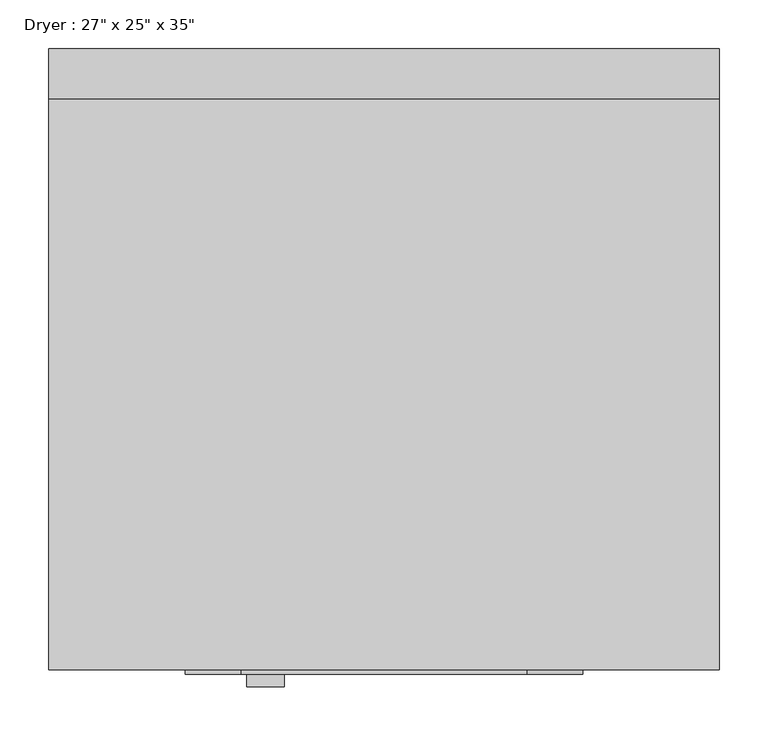
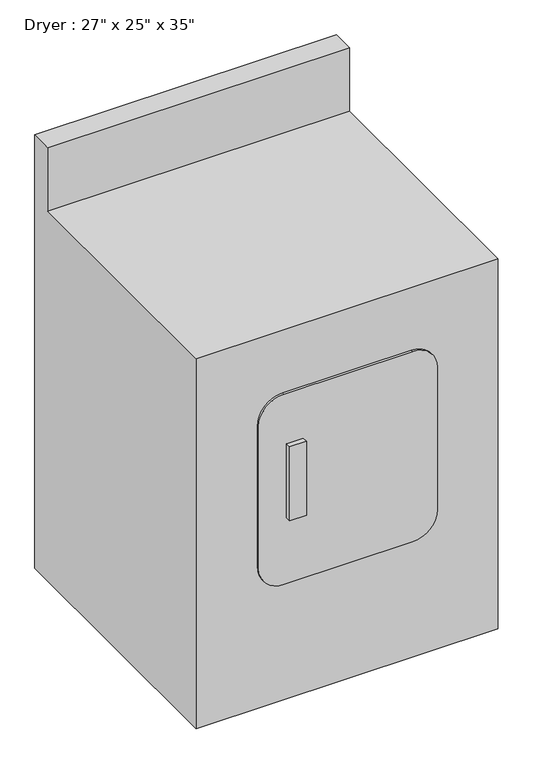
"""IFC4 building model written with IfcOpenShell, lengths in millimetres: proxy geometry."""

from ifc_helpers import new_model, si_unit, point, frame, frame_2d, origin, place, context, project, spatial, polyline, circle_curve, trimmed, segment, composite_curve, outline, extrude, source, transform, mapped, element, save


def proxy_97c73763(model_context):
    return source(origin(), model_context, "Body", "SweptSolid", [
        extrude(outline(composite_curve([segment(polyline([(737.623844, 525.0374563), (737.623844, 232.9374563)]), True, "CONTINUOUS"), segment(trimmed(circle_curve(frame_2d((680.473844, 232.9374563)), 57.15), [point((737.623844, 232.9374563))], [point((680.473844, 175.7874563))], False, "CARTESIAN"), True, "CONTINUOUS"), segment(polyline([(680.473844, 175.7874563), (337.573844, 175.7874563)]), True, "CONTINUOUS"), segment(trimmed(circle_curve(frame_2d((337.573844, 232.9374563)), 57.15), [point((337.573844, 175.7874563))], [point((280.423844, 232.9374563))], False, "CARTESIAN"), True, "CONTINUOUS"), segment(polyline([(280.423844, 232.9374563), (280.423844, 525.0374563)]), True, "CONTINUOUS"), segment(trimmed(circle_curve(frame_2d((337.573844, 525.0374563)), 57.15), [point((280.423844, 525.0374563))], [point((337.573844, 582.1874563))], False, "CARTESIAN"), True, "CONTINUOUS"), segment(polyline([(337.573844, 582.1874563), (680.473844, 582.1874563)]), True, "CONTINUOUS"), segment(trimmed(circle_curve(frame_2d((680.473844, 525.0374563)), 57.15), [point((680.473844, 582.1874563))], [point((737.623844, 525.0374563))], False, "CARTESIAN"), True, "CONTINUOUS")], self_intersect=False)), frame((0.0, -7.6014962, 0.0), z_axis=(0.0, 1.0, 0.0), x_axis=(0.0, 0.0, 1.0)), (0.0, 0.0, 1.0), 4.7625),
        extrude(outline(polyline([(276.7635206, -20.3014962), (238.6635206, -20.3014962), (238.6635206, -7.6014962), (276.7635206, -7.6014962), (276.7635206, -20.3014962)])), frame((0.0, 0.0, 438.7649313), z_axis=(0.0, 0.0, 1.0), x_axis=(1.0, 0.0, 0.0)), (0.0, 0.0, 1.0), 177.8),
        extrude(outline(polyline([(632.1610038, 0.0), (-2.8389962, 0.0), (-2.8389962, 889.0), (581.3610038, 889.0), (581.3610038, 1041.4), (632.1610038, 1041.4), (632.1610038, 0.0)])), frame((36.0874563, 0.0, 0.0), z_axis=(1.0, 0.0, 0.0), x_axis=(0.0, 1.0, 0.0)), (0.0, 0.0, 1.0), 685.8),
    ])


if __name__ == "__main__":
    model = new_model("IFC4")
    model_context = context("Model", 3, world=origin())
    ifc_project = project(units=[si_unit("LENGTHUNIT", "METRE", prefix="MILLI")], contexts=[model_context])
    site = spatial("IfcSite", under=ifc_project)
    building = spatial("IfcBuilding", under=site)
    placement = place(None, origin())
    proxy_shape = proxy_97c73763(model_context)
    element("IfcBuildingElementProxy", 1, Name="Dryer : 27\" x 25\" x 35\"", ObjectType="Dryer : 27\" x 25\" x 35\"", at=placement, inside=building, context=model_context, shape_type="MappedRepresentation", body=[
        mapped(proxy_shape, transform((0.0, 0.0, 0.0), x_axis=(1.0, 0.0, 0.0), y_axis=(0.0, 1.0, 0.0), z_axis=(0.0, 0.0, 1.0))),
    ])
    save(model, "model.ifc")

# Revit data of these elements
# Type "Dryer : 27\" x 25\" x 35\""
#   Label = "D"
#   Assembly Code = "E1090400"
#   Depth = 2' - 1"
#   Height = 2' - 11"
#   Width = 2' - 3"
#   Dryer Material = Metal - Paint Finish - Ivory,Glossy
#   Default Elevation = 0
# Element 1 (IfcBuildingElementProxy, "Dryer : 27\" x 25\" x 35\"")
#   Materials on its faces: "Metal - Paint Finish - Ivory,Glossy"
# Materials
#   "Metal - Paint Finish - Ivory,Glossy": colour RGB 247 247 239, transparency 0
